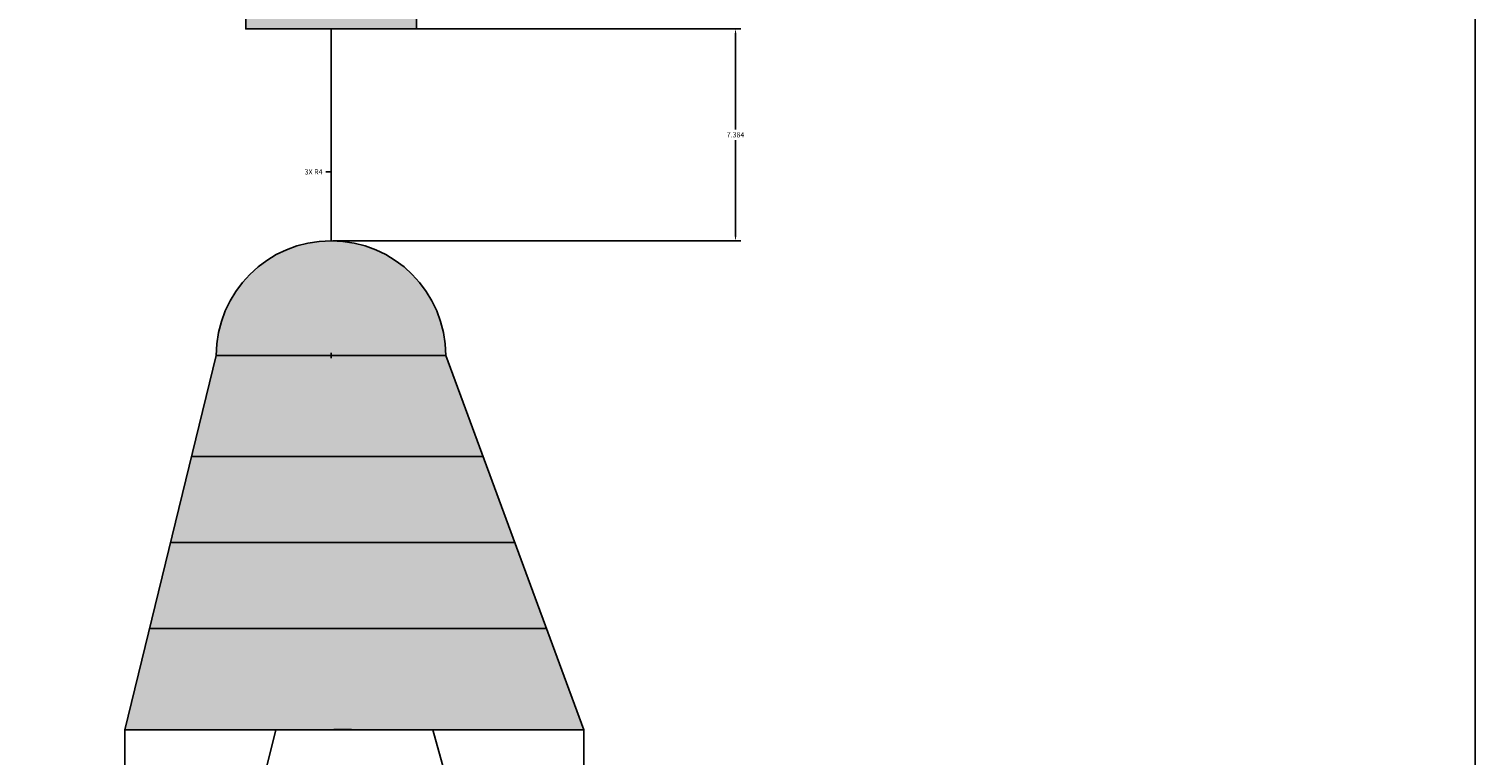
# Model space of a CAD drawing. Units: millimetres. Extents: x -8 to 285, y 5 to 221.
# Tile 29 of 30: x 221 to 271, y 166 to 191. Entities that reach past the tile are written whole.
import ezdxf

# ---------------------------------------------------------------- set-up
doc = ezdxf.new("R2010")
doc.units = ezdxf.units.MM
for name, color, linetype, lineweight in [('A-ANNO-DIMS', 2, 'Continuous', 18), ('E-EQPM-PATT', 252, 'Continuous', 13), ('E-LITE-FIXT', 7, 'Continuous', 25), ('E-LITE-SWCH', 7, 'Continuous', 25)]:
    doc.layers.add(name, color=color, linetype=linetype, lineweight=lineweight)
doc.layers.add('E-POWR-AC-LINE', color=30, linetype='Continuous', lineweight=25, true_color=0xf26722)
doc.styles.get("Standard").update_dxf_attribs({"font": 'arial.ttf'})
doc.dimstyles.get("Standard").update_dxf_attribs({"dimtxt": 0.18, "dimasz": 0.18, "dimexe": 0.18, "dimexo": 0.0625, "dimgap": 0.09, "dimtad": 0, "dimtih": 1, "dimtoh": 1, "dimdec": 4, "dimzin": 0, "dimdsep": 46, "dimtxsty": 'Standard', "dimcen": 0.09, "dimadec": 0, "dimazin": 0, "dimtfac": 1, "dimtdec": 4, "dimtofl": 0, "dimtmove": 0, "dimatfit": 3, "dimfxl": 1, "dimtolj": 1, "dimtzin": 0, "dimarcsym": 0})

# ---------------------------------------------------------------- blocks, each defined once
blk = doc.blocks.new('LAMP-INCANDESCENT')
for p, q in [((7.407, 29.994), (10.595, 43.039)), ((23.407, 29.994), (18.595, 43.039)), ((9.734, 39.517), (19.894, 39.517)), ((9.001, 36.517), (21.001, 36.517)), ((8.268, 33.517), (22.107, 33.517)), ((7.407, 29.994), (7.407, 27.935)), ((12.666, 29.994), (8.834, 14.293)), ((22.321, 14.903), (18.146, 29.994)), ((23.407, 29.994), (23.407, 27.423)), ((17.067, 15.012), (18.333, 17.205)), ((18.333, 17.205), (22.321, 14.903)), ((8.834, 14.293), (13.574, 17.029)), ((13.574, 17.029), (17.067, 15.012))]:
    blk.add_line(p, q)
for points in [[(10.595, 43.039), (18.595, 43.039)], [(23.407, 29.994), (7.407, 29.994)]]:
    blk.add_lwpolyline(points)
for centre, radius, start, end in [((14.595, 43.039), 4, 0, 180), ((15.001, 15), 15, 88.4488, 91.5512), ((15.001, 15), 15, 120.4152, 55.9163)]:
    blk.add_arc(centre, radius, start, end)
blk = doc.blocks.new('SWITCH-ON-OFF')
blk.add_line((0, 5.151), (5.948, 5.151))
blk.add_lwpolyline([(0, 10.303), (5.948, 10.303), (5.948, 0), (0, 0)], close=True)
blk = doc.blocks.new('*D9')
at = {"layer": 'A-ANNO-DIMS', "color": 0, "lineweight": -2, "transparency": 16777216}
for p, q in [((6.672, 133.79), (6.672, 220.737)), ((6.852, 220.557), (138.33, 220.557)), ((270.739, 220.557), (139.262, 220.557)), ((270.919, 206.519), (270.919, 220.737))]:
    blk.add_line(p, q, dxfattribs=at)
at = {"layer": 'A-ANNO-DIMS', "color": 0, "transparency": 16777216}
for points in [[(6.852, 220.587), (6.852, 220.527), (6.672, 220.557)], [(270.739, 220.587), (270.739, 220.527), (270.919, 220.557)]]:
    blk.add_solid(points, dxfattribs=at)
at = {"layer": 'Defpoints', "color": 0, "transparency": 16777216}
for p in [(270.919, 220.557), (270.919, 206.457), (6.672, 133.727)]:
    blk.add_point(p, dxfattribs=at)
at = {"layer": 'A-ANNO-DIMS', "color": 0, "transparency": 16777216, "insert": (138.796, 220.557), "char_height": 0.18, "attachment_point": 5}
blk.add_mtext('\\A1;264.25', dxfattribs=at)
blk = doc.blocks.new('*D16')
at = {"layer": 'A-ANNO-DIMS', "color": 0, "lineweight": -2, "transparency": 16777216}
for p, q in [((231.104, 191.491), (245.321, 191.491)), ((245.141, 191.311), (245.141, 187.981)), ((245.141, 184.287), (245.141, 187.617)), ((231.104, 184.107), (245.321, 184.107))]:
    blk.add_line(p, q, dxfattribs=at)
at = {"layer": 'A-ANNO-DIMS', "color": 0, "transparency": 16777216}
for points in [[(245.111, 191.311), (245.171, 191.311), (245.141, 191.491)], [(245.111, 184.287), (245.171, 184.287), (245.141, 184.107)]]:
    blk.add_solid(points, dxfattribs=at)
at = {"layer": 'Defpoints', "color": 0, "transparency": 16777216}
for p in [(231.041, 191.491), (231.041, 184.107), (245.141, 184.107)]:
    blk.add_point(p, dxfattribs=at)
at = {"layer": 'A-ANNO-DIMS', "color": 0, "transparency": 16777216, "insert": (245.141, 187.799), "char_height": 0.18, "attachment_point": 5}
blk.add_mtext('\\A1;7.384', dxfattribs=at)
blk = doc.blocks.new('*D30')
at = {"layer": 'A-ANNO-DIMS', "color": 0, "lineweight": -2, "transparency": 16777216}
for p, q in [((230.861, 186.507), (231.041, 186.507)), ((231.041, 186.507), (231.041, 184.287)), ((230.951, 180.107), (231.131, 180.107)), ((231.041, 180.017), (231.041, 180.197))]:
    blk.add_line(p, q, dxfattribs=at)
at = {"layer": 'A-ANNO-DIMS', "color": 0, "transparency": 16777216}
blk.add_solid([(231.071, 184.287), (231.011, 184.287), (231.041, 184.107)], dxfattribs=at)
at = {"layer": 'Defpoints', "color": 0, "transparency": 16777216}
for p in [(231.041, 184.107), (231.041, 180.107)]:
    blk.add_point(p, dxfattribs=at)
at = {"layer": 'A-ANNO-DIMS', "color": 0, "transparency": 16777216, "insert": (230.433, 186.507), "char_height": 0.18, "attachment_point": 5}
blk.add_mtext('\\A1;3X R4', dxfattribs=at)

msp = doc.modelspace()

# ---------------------------------------------------------------- hatches: boundary and pattern name
at = {"layer": 'E-EQPM-PATT'}
h = msp.add_hatch(color=256, dxfattribs=at)
h.set_gradient(color1=(254, 234, 185), color2=(254, 234, 185), tint=1)
h.paths.add_polyline_path([(148.1394, 191.4908), (148.1394, 196.6424), (142.1909, 196.6424), (142.1909, 191.4908)])
h.paths.add_polyline_path([(186.1388, 191.4908), (192.0873, 191.4908), (192.0873, 196.6424), (186.1388, 196.6424)])
h.paths.add_polyline_path([(228.067, 191.4908), (234.0155, 191.4908), (234.0155, 196.6424), (228.067, 196.6424)])
h = msp.add_hatch(color=256, dxfattribs=at)
h.set_gradient(color1=(0, 0, 255), color2=(34, 52, 110), tint=1)
h.paths.add_polyline_path([(141.2836, 180.1071), (149.2836, 180.1071, 1)])
h.paths.add_polyline_path([(149.2836, 180.1071), (141.2836, 180.1071), (140.4228, 176.5846), (150.583, 176.5846)])
h.paths.add_polyline_path([(150.583, 176.5846), (140.4228, 176.5846), (139.6897, 173.5846), (151.6897, 173.5846)])
h.paths.add_polyline_path([(151.6897, 173.5846), (139.6897, 173.5846), (138.9565, 170.5846), (152.7963, 170.5846)])
h.paths.add_polyline_path([(152.7963, 170.5846), (138.9565, 170.5846), (138.0957, 167.062), (145.2836, 167.062, -0.0135377), (146.0957, 167.062), (154.0957, 167.062)])
h.paths.add_polyline_path([(193.1131, 180.1071), (185.1131, 180.1071), (184.2522, 176.5846), (194.4125, 176.5846)])
h.paths.add_polyline_path([(185.1131, 180.1071), (193.1131, 180.1071, 1)])
h.paths.add_polyline_path([(194.4125, 176.5846), (184.2522, 176.5846), (183.5191, 173.5846), (195.5191, 173.5846)])
h.paths.add_polyline_path([(195.5191, 173.5846), (183.5191, 173.5846), (182.786, 170.5846), (196.6258, 170.5846)])
h.paths.add_polyline_path([(196.6258, 170.5846), (182.786, 170.5846), (181.9252, 167.062), (189.1131, 167.062, -0.0135377), (189.9252, 167.062), (197.9252, 167.062)])
h.paths.add_polyline_path([(227.0413, 180.1071), (235.0413, 180.1071, 1)])
h.paths.add_polyline_path([(235.0413, 180.1071), (227.0413, 180.1071), (226.1804, 176.5846), (236.3407, 176.5846)])
h.paths.add_polyline_path([(236.3407, 176.5846), (226.1804, 176.5846), (225.4473, 173.5846), (237.4473, 173.5846)])
h.paths.add_polyline_path([(237.4473, 173.5846), (225.4473, 173.5846), (224.7142, 170.5846), (238.554, 170.5846)])
h.paths.add_polyline_path([(238.554, 170.5846), (224.7142, 170.5846), (223.8534, 167.062), (231.0413, 167.062, -0.0135377), (231.8534, 167.062), (239.8534, 167.062)])
h = msp.add_hatch(color=256, dxfattribs=at)
h.set_gradient(color2=(0, 0, 0), tint=1)
h.paths.add_polyline_path([(149.2836, 180.1071, 1), (141.2836, 180.1071)])
h.paths.add_polyline_path([(193.1131, 180.1071, 1), (185.1131, 180.1071)])
h.paths.add_polyline_path([(227.0413, 180.1071), (235.0413, 180.1071, 1)])

# ---------------------------------------------------------------- linework, layer by layer
at = {"layer": 'E-POWR-AC-LINE'}
msp.add_line((231.0413, 184.1071), (231.0413, 191.4908), dxfattribs=at)
msp.add_lwpolyline([(244.6186, 34.6512), (244.6186, 49.925), (270.9192, 49.925), (270.9192, 206.4568), (145.1651, 206.4568), (145.1651, 201.7939)], dxfattribs=at)

# ---------------------------------------------------------------- block references
at = {"layer": 'E-LITE-FIXT'}
msp.add_blockref('LAMP-INCANDESCENT', (216.4466, 137.068), dxfattribs=at)
at = {"layer": 'E-LITE-SWCH'}
msp.add_blockref('SWITCH-ON-OFF', (228.0671, 191.491), dxfattribs=at)

# ---------------------------------------------------------------- dimensions: what is measured, and where the dimension line sits
at = {"layer": 'A-ANNO-DIMS'}
dim = msp.add_linear_dim(base=(270.9192, 220.5568), p1=(6.6725, 133.7273), p2=(270.9192, 206.4568), dimstyle='Standard', override={"dimdec": 2, "dimlfac": 1, "dimrnd": 0, "dimzin": 0, "dimdsep": 46, "dimlunit": 2}, dxfattribs=at)
dim.commit()
dim.dimension.update_dxf_attribs({"geometry": '*D9', "text_midpoint": (138.7958, 220.5568)})
dim = msp.add_linear_dim(base=(245.1413, 184.1071), p1=(231.0413, 191.4908), p2=(231.0413, 184.1071), angle=270, dimstyle='Standard', override={"dimdec": 3, "dimlfac": 1, "dimrnd": 0, "dimzin": 0, "dimdsep": 46, "dimlunit": 2}, dxfattribs=at)
dim.commit()
dim.dimension.update_dxf_attribs({"geometry": '*D16', "text_midpoint": (245.1413, 187.799)})
dim = msp.add_radius_dim(center=(231.0413, 180.1071), mpoint=(231.041, 184.1071), text='3X <>', dimstyle='Standard', override={"dimdec": 0, "dimlfac": 1, "dimrnd": 0, "dimzin": 0, "dimdsep": 46, "dimlunit": 2}, dxfattribs=at)
dim.commit()
dim.dimension.update_dxf_attribs({"geometry": '*D30', "text_midpoint": (230.4328, 186.5071), "dimtype": 164})

doc.saveas('drawing.dxf')
